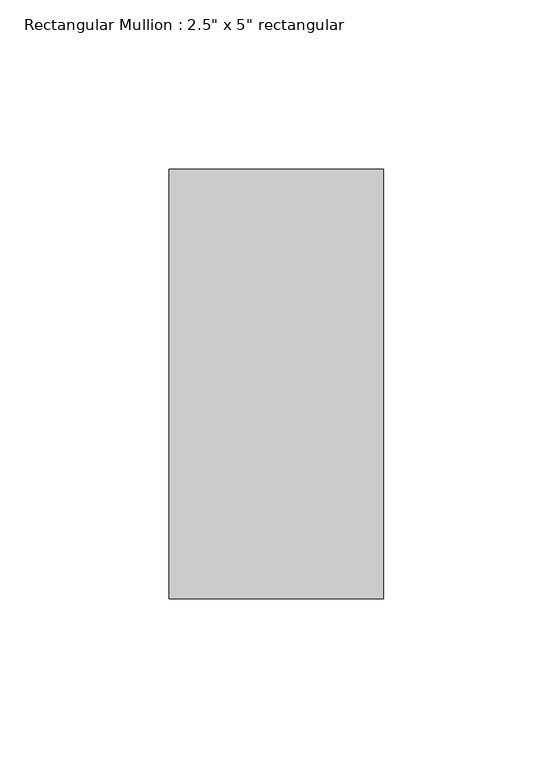
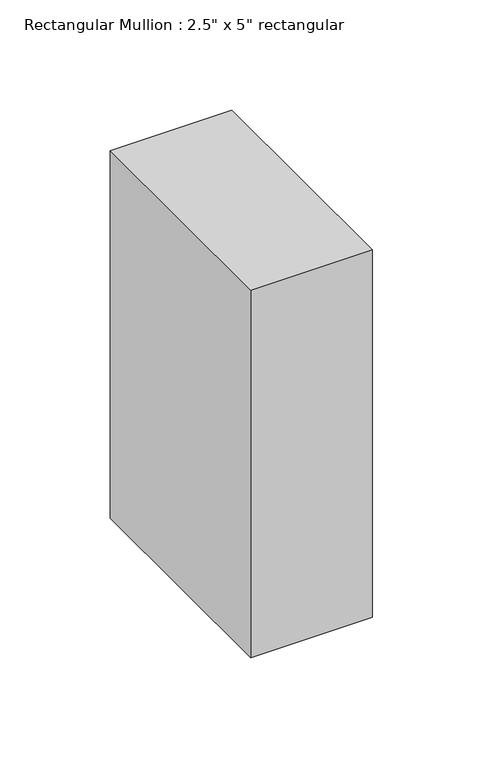
"""IFC4 building model written with IfcOpenShell, lengths in millimetres: member geometry."""

from ifc_helpers import new_model, si_unit, frame, origin, place, context, project, spatial, polyline, outline, extrude, source, transform, mapped, element, save


def member_0b6e4484(model_context):
    return source(origin(), model_context, "Body", "SweptSolid", [
        extrude(outline(polyline([(0.0, 63.5), (0.0, -63.5), (-63.5, -63.5), (-63.5, 63.5), (0.0, 63.5)])), frame((0.0, 0.0, -203.0665682), z_axis=(0.0, 0.0, 1.0), x_axis=(1.0, 0.0, 0.0)), (0.0, 0.0, 1.0), 203.0665682),
    ])


if __name__ == "__main__":
    model = new_model("IFC4")
    model_context = context("Model", 3, world=origin())
    ifc_project = project(units=[si_unit("LENGTHUNIT", "METRE", prefix="MILLI")], contexts=[model_context])
    site = spatial("IfcSite", under=ifc_project)
    building = spatial("IfcBuilding", under=site)
    placement = place(None, origin())
    member_shape = member_0b6e4484(model_context)
    element("IfcMember", 1, ObjectType="Rectangular Mullion : 2.5\" x 5\" rectangular", at=placement, inside=building, context=model_context, shape_type="MappedRepresentation", body=[
        mapped(member_shape, transform((0.0, 0.0, 0.0), x_axis=(1.0, 0.0, 0.0), y_axis=(0.0, 1.0, 0.0), z_axis=(0.0, 0.0, 1.0))),
    ])
    save(model, "model.ifc")

# Revit data of these elements
# Type "Rectangular Mullion : 2.5\" x 5\" rectangular"
#   built-in parameter 1007304 = 0.416667 (stored number, unit not read)
#   built-in parameter 1007301 = 0.104167 (stored number, unit not read)
#   built-in parameter 1007300 = 0.104167 (stored number, unit not read)
# Element 1 (IfcMember, "Rectangular Mullion : 2.5\" x 5\" rectangular")
#   Materials on its faces: "Aluminum"
# Materials
#   "Aluminum": class "Metal", colour RGB 247 247 247, transparency 0, Description = "Aluminum 6061", Cost = 0
